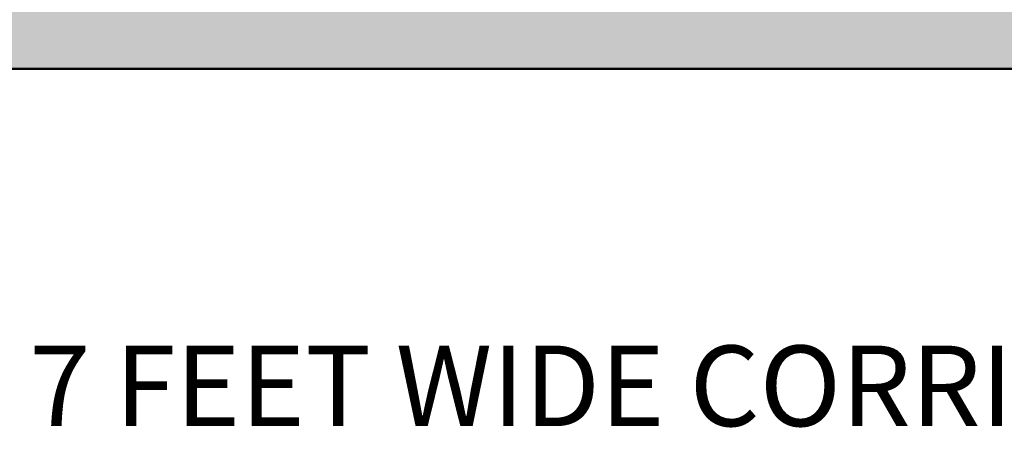
# Model space of a CAD drawing. Units: inches. Extents: x -7 to 1228, y -146 to 1091.
# Tile 59 of 88: x 429 to 531, y 531 to 573. Entities that reach past the tile are written whole.
import ezdxf

# ---------------------------------------------------------------- set-up
doc = ezdxf.new("R2010")
doc.units = ezdxf.units.IN
for name, color, linetype, lineweight in [('A-ANNO-TEXT', 7, 'Continuous', 18), ('A-WALL', 7, 'Continuous', 50), ('A-WALL-PATT', 251, 'Continuous', 13)]:
    doc.layers.add(name, color=color, linetype=linetype, lineweight=lineweight)
doc.styles.get("Standard").update_dxf_attribs({"font": 'arial.ttf'})

msp = doc.modelspace()

# ---------------------------------------------------------------- hatches: boundary and pattern name
at = {"layer": 'A-WALL-PATT'}
h = msp.add_hatch(color=256, dxfattribs=at)
h.dxf.hatch_style = 1
h.paths.add_polyline_path([(69, 568), (60, 568), (60, 493), (63.29, 493), (69, 493)])
h.paths.add_polyline_path([(69, 662.41), (60, 662.41), (60, 586), (69, 586)], flags=17)
h.paths.add_polyline_path([(69, 723), (184, 723), (184, 734), (179, 734), (179, 728), (69, 728), (69, 741.62), (60, 741.62), (60, 698.41), (69, 698.41)], flags=17)
h.paths.add_polyline_path([(69, 782), (231, 782), (231, 728), (231, 723), (231, 586), (236, 586), (236, 787), (69, 787), (69, 800.13), (60, 800.13), (60, 765.62), (69, 765.62)])
h.paths.add_polyline_path([(184, 842), (189, 842), (189, 848), (173, 848), (173, 842), (179, 842), (179, 787), (184, 787)])
h.paths.add_polyline_path([(118.22, 69), (69, 69), (69, 60), (118.22, 60)])
h.paths.add_polyline_path([(227, 69), (154.22, 69), (154.22, 60), (227, 60)])
h.paths.add_polyline_path([(236, 60), (232.71, 60), (227, 60), (227, 36), (236, 36)])
h.paths.add_polyline_path([(389, 60), (380, 60), (380, 36), (389, 36)])
h.paths.add_polyline_path([(384, 181), (380, 181), (380, 115), (380, 78), (384, 78)])
h.paths.add_polyline_path([(380, 115), (334.55, 115), (334.55, 109), (380, 109)])
h.paths.add_polyline_path([(274.55, 115), (236, 115), (236, 201), (232.71, 201), (231, 201), (231, 78), (236, 78), (236, 109), (274.55, 109)])
h.paths.add_polyline_path([(69, 123), (60, 123), (60, 78), (69, 78)])
h.paths.add_polyline_path([(69, 201), (60, 201), (60, 159), (69, 159)])
h.paths.add_polyline_path([(143, 219), (69, 219), (69, 213), (143, 213)], flags=17)
h.paths.add_polyline_path([(189, 219), (184, 219), (184, 274), (231, 274), (231, 219), (236, 219), (236, 279), (184, 279), (184, 297), (179, 297), (179, 279), (69, 279), (69, 290.91), (60, 290.91), (60, 262.18), (69, 262.18), (69, 274), (179, 274), (179, 219), (173, 219), (173, 213), (189, 213)])
h.paths.add_polyline_path([(69, 238.18), (60, 238.18), (60, 219), (69, 219)], flags=17)
h.paths.add_polyline_path([(69, 333), (60, 333), (60, 314.91), (69, 314.91), (69, 316.96)])
h.paths.add_polyline_path([(190, 338), (184, 338), (69, 338), (69, 333), (179, 333), (179, 327), (184, 327), (184, 333.02), (190, 333.05)])
h.paths.add_polyline_path([(69, 386.81), (60, 386.81), (60, 351), (69, 351)])
h.paths.add_polyline_path([(69, 475), (60, 475), (60, 422.81), (69, 422.81)])
h.paths.add_polyline_path([(236, 475), (231, 475), (231, 351.24), (236, 351.24)])
h.paths.add_polyline_path([(384, 475), (380, 475), (380, 362), (384, 362)])
h.paths.add_polyline_path([(547, 307), (439, 307), (439, 356), (445, 356), (445, 362), (433, 362), (433, 307), (380, 307), (380, 244), (380, 241), (384, 241), (384, 301), (433, 301), (433, 277), (439, 277), (439, 301), (547, 301)])
h.paths.add_polyline_path([(547, 241), (439, 241), (439, 247), (433, 247), (433, 235), (547, 235)])
h.paths.add_polyline_path([(450, 69), (440.29, 69), (424.89, 69), (389, 69), (389, 60), (450, 60)])
h.paths.add_polyline_path([(547, 69), (486, 69), (486, 60), (547, 60)])
h.paths.add_polyline_path([(556, 148.27), (547, 148.27), (547, 78), (556, 78)])
h.paths.add_polyline_path([(556, 223), (547, 223), (547, 195), (547, 184.27), (556, 184.27)])
h.paths.add_polyline_path([(556, 311.19), (547, 311.19), (547, 273.08), (556, 273.08)])
h.paths.add_polyline_path([(556, 344), (552.71, 344), (547, 344), (547, 335.19), (556, 335.19)])
h.paths.add_polyline_path([(556, 249.08), (547, 249.08), (547, 241), (556, 241)])
h.paths.add_polyline_path([(547, 362), (475, 362), (475, 356), (547, 356)], flags=0)
h.paths.add_polyline_path([(556, 399.62), (547, 399.62), (547, 362), (556, 362)])
h.paths.add_polyline_path([(556, 475), (547, 475), (547, 435.62), (556, 435.62)])
h.paths.add_polyline_path([(547, 493), (389, 493), (389, 487), (547, 487)])
h.paths.add_polyline_path([(380, 493), (278, 493), (278, 487), (380, 487)])
h.paths.add_polyline_path([(227, 493), (69, 493), (69, 487), (227, 487)])
h.paths.add_polyline_path([(643, 122.44), (634, 122.44), (634, 78), (643, 78)])
h.paths.add_polyline_path([(702.5, 69), (692.79, 69), (677.39, 69), (643, 69), (643, 60), (702.5, 60)])
h.paths.add_polyline_path([(798, 69), (738.5, 69), (738.5, 60), (798, 60)])
h.paths.add_polyline_path([(807, 60), (803.71, 60), (798, 60), (798, 36), (807, 36)])
h.paths.add_polyline_path([(807, 109), (846.75, 109), (846.75, 115), (807, 115), (807, 159), (802, 159), (802, 78), (807, 78)])
h.paths.add_polyline_path([(807, 201), (802, 201), (802, 195), (807, 195)])
h.paths.add_polyline_path([(643, 201), (634, 201), (634, 158.44), (643, 158.44)])
h.paths.add_polyline_path([(756, 225), (751, 225), (751, 219), (643, 219), (643, 213), (756, 213)])
h.paths.add_polyline_path([(643, 240.85), (634, 240.85), (634, 219), (643, 219)])
h.paths.add_polyline_path([(643, 274), (643, 288.63), (634, 288.63), (634, 264.85), (643, 264.85)])
h.paths.add_polyline_path([(802, 279), (756, 279), (756, 297), (751, 297), (751, 279), (643, 279), (643, 274), (751, 274), (751, 255), (756, 255), (756, 274), (802, 274)])
h.paths.add_polyline_path([(807, 333), (803.71, 333), (802, 333), (802, 279), (802, 274), (802, 219), (807, 219)])
h.paths.add_polyline_path([(956, 182), (951, 182), (951, 115), (906.75, 115), (906.75, 109), (951, 109), (951, 78), (956, 78)])
h.paths.add_polyline_path([(960, 60), (951, 60), (951, 36), (960, 36)])
h.paths.add_polyline_path([(1021, 69), (1005.78, 69), (960, 69), (960, 60), (1021, 60)])
h.paths.add_polyline_path([(956, 224), (951, 224), (951, 218), (956, 218)])
h.paths.add_polyline_path([(956, 302), (1004, 302), (1004, 278), (1010, 278), (1010, 302), (1118, 302), (1118, 290.81), (1127, 290.81), (1127, 326.97), (1118, 326.97), (1118, 320.97), (1118, 307), (1010, 307), (1010, 356), (1016, 356), (1016, 362), (1004, 362), (1004, 307), (951, 307), (951, 244), (951, 242), (954.29, 242), (956, 242)])
h.paths.add_polyline_path([(643, 333), (634, 333), (634, 312.63), (643, 312.63), (643, 316.96)])
h.paths.add_polyline_path([(756, 338), (643, 338), (643, 333), (751, 333), (751, 327), (756, 327)])
h.paths.add_polyline_path([(643, 388), (634, 388), (634, 351), (643, 351)])
h.paths.add_polyline_path([(807, 357), (802, 357), (802, 351), (807, 351)])
h.paths.add_polyline_path([(807, 475), (802, 475), (802, 393), (807, 393)])
h.paths.add_polyline_path([(643, 475), (634, 475), (634, 424), (643, 424)])
h.paths.add_polyline_path([(798, 493), (643, 493), (643, 487), (798, 487)])
h.paths.add_polyline_path([(634, 493), (556, 493), (556, 487), (634, 487)])
h.paths.add_polyline_path([(813, 493), (807, 493), (807, 487), (813, 487)])
h.paths.add_polyline_path([(951, 493), (849, 493), (849, 487), (951, 487)])
h.paths.add_polyline_path([(956, 484), (951, 484), (951, 374), (956, 374)])
h.paths.add_polyline_path([(1109, 493), (969, 493), (969, 487), (1109, 487)])
h.paths.add_polyline_path([(1127, 484), (1118, 484), (1118, 450.64), (1127, 450.64)])
h.paths.add_polyline_path([(1127, 414.64), (1118, 414.64), (1118, 365), (1127, 365)])
h.paths.add_polyline_path([(1109, 362), (1046, 362), (1046, 356), (1109, 356)], flags=17)
h.paths.add_polyline_path([(1127, 356), (1123.45, 356), (1118, 356), (1118, 350.97), (1127, 350.97)], flags=0)
h.paths.add_polyline_path([(1127, 266.81), (1118, 266.81), (1118, 262.36), (1118, 242), (1127, 242)], flags=17)
h.paths.add_polyline_path([(1118, 242), (1010, 242), (1010, 248), (1004, 248), (1004, 237), (1118, 237)])
h.paths.add_polyline_path([(1127, 224), (1118, 224), (1118, 170), (1127, 170)])
h.paths.add_polyline_path([(1127, 134), (1118, 134), (1118, 78), (1127, 78)])
h.paths.add_polyline_path([(1118, 69), (1057, 69), (1057, 60), (1118, 60)])
h.paths.add_polyline_path([(227, 571.55), (227, 574), (69, 574), (69, 568), (227, 568)])
h.paths.add_polyline_path([(380, 571.55), (380, 574), (278, 574), (278, 568), (380, 568)])
h.paths.add_polyline_path([(242, 574), (236, 574), (236, 568), (242, 568)])
h.paths.add_polyline_path([(547, 571.55), (547, 574), (389, 574), (389, 568), (547, 568)])
h.paths.add_polyline_path([(384, 733), (380, 733), (380, 586), (384, 586)])
h.paths.add_polyline_path([(556, 646), (634, 646), (634, 655), (547, 655), (547, 586), (556, 586)])
h.paths.add_polyline_path([(634, 574), (556, 574), (556, 568), (634, 568)])
h.paths.add_polyline_path([(643, 655), (634, 655), (634, 586), (643, 586)])
h.paths.add_polyline_path([(798, 574), (643, 574), (643, 568), (798, 568)])
h.paths.add_polyline_path([(643, 663.85), (634, 663.85), (634, 655), (643, 655)])
h.paths.add_polyline_path([(556, 676.97), (547, 676.97), (547, 655), (556, 655)])
h.paths.add_polyline_path([(556, 733), (547, 733), (547, 712.97), (556, 712.97)])
h.paths.add_polyline_path([(643, 710), (634, 710), (634, 699.85), (643, 699.85)])
h.paths.add_polyline_path([(807, 668), (802, 668), (802, 586), (807, 586)])
h.paths.add_polyline_path([(951, 574), (849, 574), (849, 568), (951, 568)])
h.paths.add_polyline_path([(956, 691), (951, 691), (951, 577), (956, 577)])
h.paths.add_polyline_path([(1109, 574), (969, 574), (969, 568), (1109, 568)])
h.paths.add_polyline_path([(1127, 643.4), (1118, 643.4), (1118, 577), (1127, 577)])
h.paths.add_polyline_path([(1127, 568), (1123.45, 568), (1118, 568), (1118, 493), (1127, 493)])
h.paths.add_polyline_path([(1127, 733), (1118, 733), (1118, 679.4), (1127, 679.4)])
h.paths.add_polyline_path([(1127, 777.35), (1118, 777.35), (1118, 770.04), (1118, 751), (1127, 751)], flags=17)
h.paths.add_polyline_path([(1118, 751), (1010, 751), (1010, 757), (1004, 757), (1004, 745), (1118, 745)])
h.paths.add_polyline_path([(956, 811), (1004, 811), (1004, 787), (1010, 787), (1010, 811), (1017.87, 811), (1017.87, 811.63, -0.414214), (1018.25, 812), (1031.98, 812, -0.414214), (1032.35, 811.63), (1032.35, 811), (1118, 811), (1118, 801.35), (1127, 801.35), (1127, 834.69), (1118, 834.69), (1118, 830.24), (1118, 817), (1010, 817), (1010, 866), (1016, 866), (1016, 872), (1004, 872), (1004, 817), (956, 817), (956, 866), (951, 866), (951, 751), (954.29, 751), (956, 751)])
h.paths.add_polyline_path([(1118, 872), (1046, 872), (1046, 866), (1118, 866)], flags=17)
h.paths.add_polyline_path([(1127, 924.71), (1118, 924.71), (1118, 884), (1127, 884)])
h.paths.add_polyline_path([(1127, 866), (1123.71, 866), (1118, 866), (1118, 858.69), (1127, 858.69)], flags=17)
h.paths.add_polyline_path([(956, 983), (951, 983), (951, 952), (807, 952), (807, 983), (802, 983), (802, 902), (807, 902), (807, 946), (951, 946), (951, 884), (956, 884)])
h.paths.add_polyline_path([(807, 842), (802, 842), (802, 787), (756, 787), (756, 806), (751, 806), (751, 787), (643, 787), (643, 782), (751, 782), (751, 764), (756, 764), (756, 782), (802, 782), (802, 728), (807, 728)])
h.paths.add_polyline_path([(756, 848), (643, 848), (643, 842), (751, 842), (751, 836), (756, 836)])
h.paths.add_polyline_path([(756, 734), (751, 734), (751, 728), (643, 728), (643, 723), (756, 723)])
h.paths.add_polyline_path([(643, 749.79), (634, 749.79), (634, 728), (637.29, 728), (643, 728)])
h.paths.add_polyline_path([(643, 805.41), (634, 805.41), (634, 773.79), (643, 773.79)])
h.paths.add_polyline_path([(643, 896.66), (634, 896.66), (634, 860), (637.29, 860), (643, 860)])
h.paths.add_polyline_path([(643, 842), (634, 842), (634, 829.41), (643, 829.41)])
h.paths.add_polyline_path([(643, 983), (634, 983), (634, 932.66), (643, 932.66)])
h.paths.add_polyline_path([(1127, 983), (1118, 983), (1118, 960.71), (1127, 960.71)])
h.paths.add_polyline_path([(1118, 1001), (1077.53, 1001), (1077.53, 992), (1118, 992)])
h.paths.add_polyline_path([(1041.53, 1001), (960, 1001), (960, 992), (1041.53, 992)])
h.paths.add_polyline_path([(960, 1025), (951, 1025), (951, 1001), (954.29, 1001), (960, 1001)])
h.paths.add_polyline_path([(807, 1025), (798, 1025), (798, 1001), (807, 1001)])
h.paths.add_polyline_path([(798, 1001), (738.5, 1001), (738.5, 992), (798, 992)])
h.paths.add_polyline_path([(702.5, 1001), (643, 1001), (643, 992), (702.5, 992)])
h.paths.add_polyline_path([(547, 1001), (499.11, 1001), (499.11, 992), (547, 992)])
h.paths.add_polyline_path([(463.11, 1001), (389, 1001), (389, 992), (463.11, 992)])
h.paths.add_polyline_path([(389, 1025), (380, 1025), (380, 1022), (380, 1001), (383.29, 1001), (389, 1001)])
h.paths.add_polyline_path([(236, 1025), (227, 1025), (227, 1001), (236, 1001)])
h.paths.add_polyline_path([(236, 983), (231, 983), (231, 860), (236, 860)])
h.paths.add_polyline_path([(274.55, 952), (236, 952), (236, 946), (274.55, 946)])
h.paths.add_polyline_path([(380, 952), (334.55, 952), (334.55, 946), (380, 946)])
h.paths.add_polyline_path([(384, 983), (380, 983), (380, 884), (383.29, 884), (384, 884)])
h.paths.add_polyline_path([(227, 1001), (155.01, 1001), (155.01, 992), (162.87, 992), (227, 992)])
h.paths.add_polyline_path([(119.01, 1001), (69, 1001), (69, 992), (119.01, 992)])
h.paths.add_polyline_path([(69, 983), (60, 983), (60, 922.99), (69, 922.99)])
h.paths.add_polyline_path([(69, 886.99), (60, 886.99), (60, 860), (63.29, 860), (69, 860)])
h.paths.add_polyline_path([(143, 848), (69, 848), (69, 842), (143, 842)])

# ---------------------------------------------------------------- linework, layer by layer
at = {"layer": 'A-WALL'}
msp.add_line((547, 568), (384, 568), dxfattribs=at)

# ---------------------------------------------------------------- texts
at = {"layer": 'A-ANNO-TEXT', "insert": (430.35, 539.42), "char_height": 8.3203, "attachment_point": 1}
msp.add_mtext_dynamic_manual_height_columns('7 FEET WIDE CORRIDOR', width=225.8822, gutter_width=41.6, heights=[0], dxfattribs=at)

doc.saveas('drawing.dxf')
